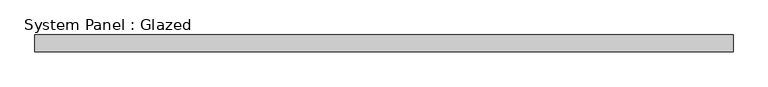
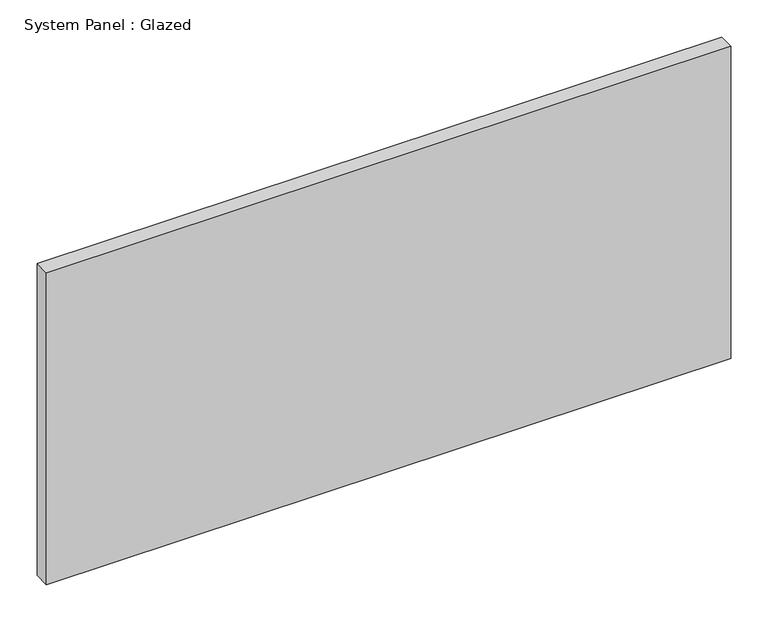
"""IFC4 building model written with IfcOpenShell, lengths in millimetres: plate geometry, System Panel : Glazed."""

from ifc_helpers import new_model, si_unit, origin, origin_with_axes, place, context, project, spatial, polyline, outline, extrude, source, transform, mapped, element, save


def system_panel_glazed_ef7cd4ce(model_context):
    return source(origin(), model_context, "Body", "SweptSolid", [
        extrude(outline(polyline([(533.4, 19.05), (-533.4, 19.05), (-533.4, 44.45), (533.4, 44.45), (533.4, 19.05)])), origin_with_axes(), (0.0, 0.0, 1.0), 514.35),
    ])


if __name__ == "__main__":
    model = new_model("IFC4")
    model_context = context("Model", 3, world=origin())
    ifc_project = project(units=[si_unit("LENGTHUNIT", "METRE", prefix="MILLI")], contexts=[model_context])
    site = spatial("IfcSite", under=ifc_project)
    building = spatial("IfcBuilding", under=site)
    placement = place(None, origin())
    system_panel_glazed_shape = system_panel_glazed_ef7cd4ce(model_context)
    element("IfcPlate", 1, ObjectType="System Panel : Glazed", at=placement, inside=building, context=model_context, shape_type="MappedRepresentation", body=[
        mapped(system_panel_glazed_shape, transform((0.0, 0.0, 0.0), x_axis=(1.0, 0.0, 0.0), y_axis=(0.0, 1.0, 0.0), z_axis=(0.0, 0.0, 1.0))),
    ])
    save(model, "model.ifc")

# Revit data of these elements
# Type "System Panel : Glazed"
#   Construction Type Id = "GSP4R"
#   Analytic Construction = "1/8 in Pilkington single glazing"
#   Visual Light Transmittance = 0.9
#   Solar Heat Gain Coefficient = 0.86
#   Heat Transfer Coefficient (U) = 1.18115 BTU/(h·ft²·°F)
#   Define Thermal Properties by = 1
# Element 1 (IfcPlate, "System Panel : Glazed")
#   Materials on its faces: "Glass"
# Materials
#   "Glass": class "Glass", colour RGB 0 128 192, transparency 0.75, Description = "Soda Lime Glass", Cost = 0
